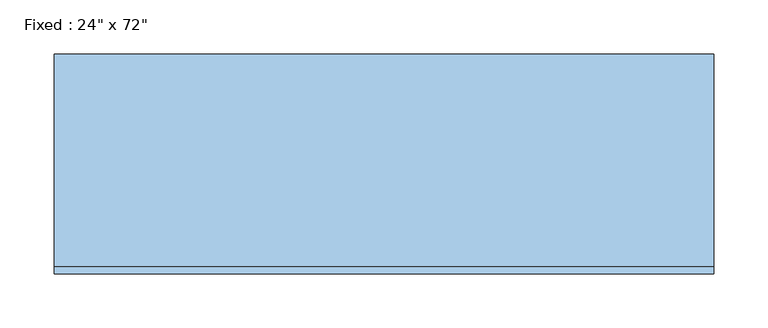
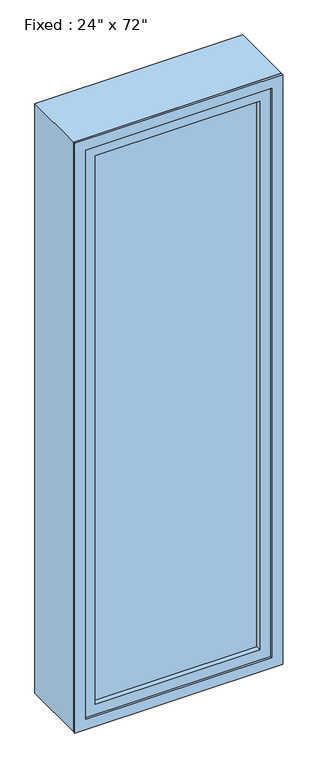
"""IFC4 building model written with IfcOpenShell, lengths in millimetres: window geometry."""

from ifc_helpers import new_model, si_unit, frame, origin, place, context, project, spatial, polyline, outline, extrude, source, transform, mapped, element, save


def window_a028c9d7(model_context):
    return source(origin(), model_context, "Body", "SweptSolid", [
        extrude(outline(polyline([(203.2, -79.375), (-279.4, -79.375), (-279.4, -66.675), (203.2, -66.675), (203.2, -79.375)])), frame((0.0, 0.0, 368.3), z_axis=(0.0, 0.0, 1.0), x_axis=(1.0, 0.0, 0.0)), (0.0, 0.0, 1.0), 1701.8),
        extrude(outline(polyline([(2114.55, -323.85), (323.85, -323.85), (323.85, 247.65), (2114.55, 247.65), (2114.55, -323.85)]), holes=[polyline([(2070.1, -279.4), (2070.1, 203.2), (368.3, 203.2), (368.3, -279.4), (2070.1, -279.4)])]), frame((0.0, -95.25, 0.0), z_axis=(0.0, 1.0, 0.0), x_axis=(0.0, 0.0, 1.0)), (0.0, 0.0, 1.0), 44.45),
        extrude(outline(polyline([(2133.6, -342.9), (304.8, -342.9), (304.8, 266.7), (2133.6, 266.7), (2133.6, -342.9)]), holes=[polyline([(2101.85, -311.15), (2101.85, 234.95), (336.55, 234.95), (336.55, -311.15), (2101.85, -311.15)])]), frame((0.0, -101.6, 0.0), z_axis=(0.0, 1.0, 0.0), x_axis=(0.0, 0.0, 1.0)), (0.0, 0.0, 1.0), 6.35),
        extrude(outline(polyline([(2133.6, 266.7), (2133.6, -342.9), (304.8, -342.9), (304.8, 266.7), (2133.6, 266.7)]), holes=[polyline([(2114.55, 247.65), (323.85, 247.65), (323.85, -323.85), (2114.55, -323.85), (2114.55, 247.65)])]), frame((0.0, -95.25, 0.0), z_axis=(0.0, 1.0, 0.0), x_axis=(0.0, 0.0, 1.0)), (0.0, 0.0, 1.0), 196.85),
    ])


if __name__ == "__main__":
    model = new_model("IFC4")
    model_context = context("Model", 3, world=origin())
    ifc_project = project(units=[si_unit("LENGTHUNIT", "METRE", prefix="MILLI")], contexts=[model_context])
    site = spatial("IfcSite", under=ifc_project)
    building = spatial("IfcBuilding", under=site)
    placement = place(None, origin())
    window_shape = window_a028c9d7(model_context)
    element("IfcWindow", 1, ObjectType="Fixed : 24\" x 72\"", at=placement, inside=building, context=model_context, shape_type="MappedRepresentation", body=[
        mapped(window_shape, transform((0.0, 0.0, 0.0), x_axis=(1.0, 0.0, 0.0), y_axis=(0.0, 1.0, 0.0), z_axis=(0.0, 0.0, 1.0))),
    ])
    save(model, "model.ifc")

# Revit data of these elements
# Type "Fixed : 24\" x 72\""
#   Type Mark = "14"
#   Construction Type Id = "GSP4R"
#   Assembly Code = "B2020100"
#   Analytic Construction = "1/8 in Pilkington single glazing"
#   Visual Light Transmittance = 0.9
#   Solar Heat Gain Coefficient = 0.78
#   Heat Transfer Coefficient (U) = 0.6496 BTU/(h·ft²·°F)
#   Height = 6' - 0"
#   Default Sill Height = 1' - 0"
#   Width = 2' - 0"
#   Window Inset = 0' - 6"
#   Define Thermal Properties by = 1
#   Glass Pane Material = Glass
#   Sash Material = Structure, Steel Bar Joist Layer
#   Wall Closure = (empty or 0)
# Element 1 (IfcWindow, "Fixed : 24\" x 72\"")
#   Materials on its faces: "Structure, Steel Bar Joist Layer", "Glass"
# Materials
#   "Glass": class "Glass", colour RGB 0 128 192, transparency 0.75, Description = "Soda Lime Glass", Cost = 0
#   "Structure, Steel Bar Joist Layer": class "Metal", colour RGB 127 127 127, transparency 0, Description = "Bar joists, thermal airspace", Cost = 0
